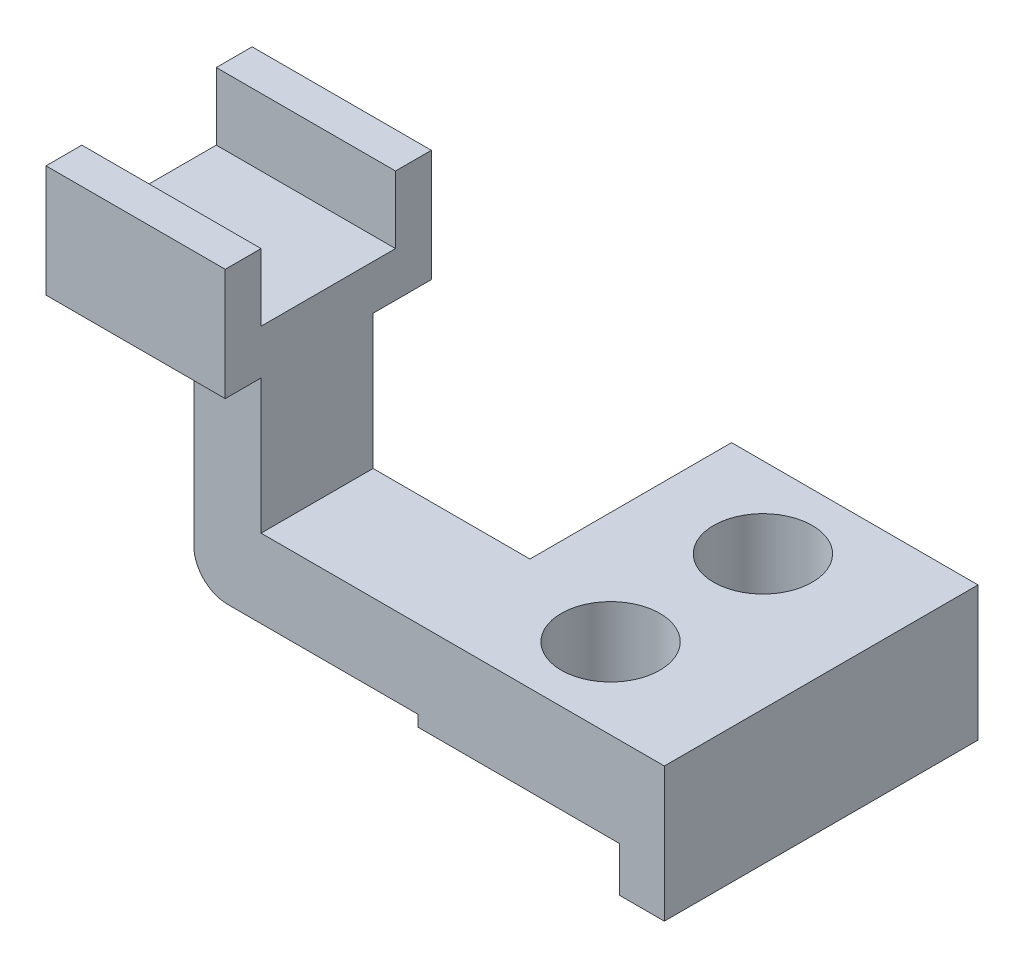
ISO-10303-21;
HEADER;
FILE_DESCRIPTION(('STEP AP214'),'2;1');
FILE_NAME('part.step','',(''),(''),'','','');
FILE_SCHEMA(('AUTOMOTIVE_DESIGN { 1 0 10303 214 1 1 1 1 }'));
ENDSEC;
DATA;
#1=APPLICATION_CONTEXT('core data for automotive mechanical design processes');
#2=APPLICATION_PROTOCOL_DEFINITION('international standard','automotive_design',2000,#1);
#3=PRODUCT_CONTEXT('',#1,'mechanical');
#4=PRODUCT('Part','Part','',(#3));
#5=PRODUCT_RELATED_PRODUCT_CATEGORY('part','',(#4));
#6=PRODUCT_DEFINITION_FORMATION('','',#4);
#7=PRODUCT_DEFINITION_CONTEXT('part definition',#1,'design');
#8=PRODUCT_DEFINITION('design','',#6,#7);
#9=PRODUCT_DEFINITION_SHAPE('','',#8);
#10=(LENGTH_UNIT() NAMED_UNIT(*) SI_UNIT(.MILLI.,.METRE.));
#11=(NAMED_UNIT(*) PLANE_ANGLE_UNIT() SI_UNIT($,.RADIAN.));
#12=(NAMED_UNIT(*) SI_UNIT($,.STERADIAN.) SOLID_ANGLE_UNIT());
#13=UNCERTAINTY_MEASURE_WITH_UNIT(LENGTH_MEASURE(1.E-05),#10,'distance_accuracy_value','');
#14=(GEOMETRIC_REPRESENTATION_CONTEXT(3) GLOBAL_UNCERTAINTY_ASSIGNED_CONTEXT((#13)) GLOBAL_UNIT_ASSIGNED_CONTEXT((#10,
#11,#12)) REPRESENTATION_CONTEXT('',''));
#15=CARTESIAN_POINT('',(0.,0.,0.));
#16=DIRECTION('',(0.,0.,1.));
#17=DIRECTION('',(1.,0.,0.));
#18=AXIS2_PLACEMENT_3D('',#15,#16,#17);
#19=CARTESIAN_POINT('',(0.,20.,70.));
#20=DIRECTION('',(1.,0.,0.));
#21=DIRECTION('',(0.,0.,-1.));
#22=AXIS2_PLACEMENT_3D('',#19,#20,#21);
#23=PLANE('',#22);
#24=DIRECTION('',(0.,0.,1.));
#25=VECTOR('',#24,1.);
#26=CARTESIAN_POINT('',(0.,2.5,45.));
#27=LINE('',#26,#25);
#28=CARTESIAN_POINT('',(0.,2.5,45.));
#29=VERTEX_POINT('',#28);
#30=CARTESIAN_POINT('',(0.,2.5,70.));
#31=VERTEX_POINT('',#30);
#32=EDGE_CURVE('E305',#29,#31,#27,.T.);
#33=ORIENTED_EDGE('',*,*,#32,.F.);
#34=DIRECTION('',(0.,-1.,0.));
#35=VECTOR('',#34,1.);
#36=CARTESIAN_POINT('',(0.,0.,45.));
#37=LINE('',#36,#35);
#38=CARTESIAN_POINT('',(0.,20.,45.));
#39=VERTEX_POINT('',#38);
#40=EDGE_CURVE('E63',#39,#29,#37,.T.);
#41=ORIENTED_EDGE('',*,*,#40,.F.);
#42=DIRECTION('',(0.,0.,-1.));
#43=VECTOR('',#42,1.);
#44=CARTESIAN_POINT('',(0.,20.,70.));
#45=LINE('',#44,#43);
#46=CARTESIAN_POINT('',(0.,20.,0.));
#47=VERTEX_POINT('',#46);
#48=EDGE_CURVE('E317',#39,#47,#45,.T.);
#49=ORIENTED_EDGE('',*,*,#48,.T.);
#50=DIRECTION('',(0.,-1.,0.));
#51=VECTOR('',#50,1.);
#52=CARTESIAN_POINT('',(0.,20.,0.));
#53=LINE('',#52,#51);
#54=CARTESIAN_POINT('',(0.,0.,0.));
#55=VERTEX_POINT('',#54);
#56=EDGE_CURVE('E296',#47,#55,#53,.T.);
#57=ORIENTED_EDGE('',*,*,#56,.T.);
#58=DIRECTION('',(0.,0.,-1.));
#59=VECTOR('',#58,1.);
#60=CARTESIAN_POINT('',(0.,0.,70.));
#61=LINE('',#60,#59);
#62=CARTESIAN_POINT('',(0.,0.,70.));
#63=VERTEX_POINT('',#62);
#64=EDGE_CURVE('E11',#63,#55,#61,.T.);
#65=ORIENTED_EDGE('',*,*,#64,.F.);
#66=DIRECTION('',(0.,-1.,0.));
#67=VECTOR('',#66,1.);
#68=CARTESIAN_POINT('',(0.,20.,70.));
#69=LINE('',#68,#67);
#70=EDGE_CURVE('E70',#31,#63,#69,.T.);
#71=ORIENTED_EDGE('',*,*,#70,.F.);
#72=EDGE_LOOP('',(#33,#41,#49,#57,#65,#71));
#73=FACE_BOUND('',#72,.T.);
#74=ADVANCED_FACE('F50',(#73),#23,.F.);
#75=CARTESIAN_POINT('',(0.,0.,70.));
#76=DIRECTION('',(0.,1.,0.));
#77=DIRECTION('',(0.,0.,1.));
#78=AXIS2_PLACEMENT_3D('',#75,#76,#77);
#79=PLANE('',#78);
#80=CARTESIAN_POINT('',(25.,0.,18.));
#81=DIRECTION('',(0.,1.,0.));
#82=DIRECTION('',(0.,0.,1.));
#83=AXIS2_PLACEMENT_3D('',#80,#81,#82);
#84=CIRCLE('',#83,11.);
#85=CARTESIAN_POINT('',(25.,0.,29.));
#86=VERTEX_POINT('',#85);
#87=EDGE_CURVE('E216',#86,#86,#84,.T.);
#88=ORIENTED_EDGE('',*,*,#87,.T.);
#89=EDGE_LOOP('',(#88));
#90=FACE_BOUND('',#89,.T.);
#91=CARTESIAN_POINT('',(25.,0.,52.));
#92=DIRECTION('',(0.,1.,0.));
#93=DIRECTION('',(0.,0.,1.));
#94=AXIS2_PLACEMENT_3D('',#91,#92,#93);
#95=CIRCLE('',#94,11.);
#96=CARTESIAN_POINT('',(25.,0.,63.));
#97=VERTEX_POINT('',#96);
#98=EDGE_CURVE('E732',#97,#97,#95,.T.);
#99=ORIENTED_EDGE('',*,*,#98,.T.);
#100=EDGE_LOOP('',(#99));
#101=FACE_BOUND('',#100,.T.);
#102=DIRECTION('',(1.,0.,0.));
#103=VECTOR('',#102,1.);
#104=CARTESIAN_POINT('',(0.,0.,0.));
#105=LINE('',#104,#103);
#106=CARTESIAN_POINT('',(45.,0.,0.));
#107=VERTEX_POINT('',#106);
#108=EDGE_CURVE('E325',#55,#107,#105,.T.);
#109=ORIENTED_EDGE('',*,*,#108,.T.);
#110=DIRECTION('',(0.,0.,-1.));
#111=VECTOR('',#110,1.);
#112=CARTESIAN_POINT('',(45.,0.,70.));
#113=LINE('',#112,#111);
#114=CARTESIAN_POINT('',(45.,0.,70.));
#115=VERTEX_POINT('',#114);
#116=EDGE_CURVE('E53',#115,#107,#113,.T.);
#117=ORIENTED_EDGE('',*,*,#116,.F.);
#118=DIRECTION('',(1.,0.,0.));
#119=VECTOR('',#118,1.);
#120=CARTESIAN_POINT('',(0.,0.,70.));
#121=LINE('',#120,#119);
#122=EDGE_CURVE('E306',#63,#115,#121,.T.);
#123=ORIENTED_EDGE('',*,*,#122,.F.);
#124=ORIENTED_EDGE('',*,*,#64,.T.);
#125=EDGE_LOOP('',(#109,#117,#123,#124));
#126=FACE_BOUND('',#125,.T.);
#127=ADVANCED_FACE('F366',(#90,#101,#126),#79,.F.);
#128=CARTESIAN_POINT('',(45.,0.,70.));
#129=DIRECTION('',(1.,0.,0.));
#130=DIRECTION('',(0.,0.,-1.));
#131=AXIS2_PLACEMENT_3D('',#128,#129,#130);
#132=PLANE('',#131);
#133=DIRECTION('',(0.,-1.,0.));
#134=VECTOR('',#133,1.);
#135=CARTESIAN_POINT('',(45.,0.,0.));
#136=LINE('',#135,#134);
#137=CARTESIAN_POINT('',(45.,-10.,0.));
#138=VERTEX_POINT('',#137);
#139=EDGE_CURVE('E322',#107,#138,#136,.T.);
#140=ORIENTED_EDGE('',*,*,#139,.T.);
#141=DIRECTION('',(0.,0.,-1.));
#142=VECTOR('',#141,1.);
#143=CARTESIAN_POINT('',(45.,-10.,70.));
#144=LINE('',#143,#142);
#145=CARTESIAN_POINT('',(45.,-10.,70.));
#146=VERTEX_POINT('',#145);
#147=EDGE_CURVE('E339',#146,#138,#144,.T.);
#148=ORIENTED_EDGE('',*,*,#147,.F.);
#149=DIRECTION('',(0.,-1.,0.));
#150=VECTOR('',#149,1.);
#151=CARTESIAN_POINT('',(45.,0.,70.));
#152=LINE('',#151,#150);
#153=EDGE_CURVE('E313',#115,#146,#152,.T.);
#154=ORIENTED_EDGE('',*,*,#153,.F.);
#155=ORIENTED_EDGE('',*,*,#116,.T.);
#156=EDGE_LOOP('',(#140,#148,#154,#155));
#157=FACE_BOUND('',#156,.T.);
#158=ADVANCED_FACE('F347',(#157),#132,.F.);
#159=CARTESIAN_POINT('',(45.,-10.,70.));
#160=DIRECTION('',(0.,1.,0.));
#161=DIRECTION('',(0.,0.,1.));
#162=AXIS2_PLACEMENT_3D('',#159,#160,#161);
#163=PLANE('',#162);
#164=DIRECTION('',(1.,0.,0.));
#165=VECTOR('',#164,1.);
#166=CARTESIAN_POINT('',(45.,-10.,0.));
#167=LINE('',#166,#165);
#168=CARTESIAN_POINT('',(55.,-10.,0.));
#169=VERTEX_POINT('',#168);
#170=EDGE_CURVE('E326',#138,#169,#167,.T.);
#171=ORIENTED_EDGE('',*,*,#170,.T.);
#172=DIRECTION('',(0.,0.,-1.));
#173=VECTOR('',#172,1.);
#174=CARTESIAN_POINT('',(55.,-10.,70.));
#175=LINE('',#174,#173);
#176=CARTESIAN_POINT('',(55.,-10.,70.));
#177=VERTEX_POINT('',#176);
#178=EDGE_CURVE('E338',#177,#169,#175,.T.);
#179=ORIENTED_EDGE('',*,*,#178,.F.);
#180=DIRECTION('',(1.,0.,0.));
#181=VECTOR('',#180,1.);
#182=CARTESIAN_POINT('',(45.,-10.,70.));
#183=LINE('',#182,#181);
#184=EDGE_CURVE('E311',#146,#177,#183,.T.);
#185=ORIENTED_EDGE('',*,*,#184,.F.);
#186=ORIENTED_EDGE('',*,*,#147,.T.);
#187=EDGE_LOOP('',(#171,#179,#185,#186));
#188=FACE_BOUND('',#187,.T.);
#189=ADVANCED_FACE('F356',(#188),#163,.F.);
#190=CARTESIAN_POINT('',(55.,-10.,70.));
#191=DIRECTION('',(-1.,0.,0.));
#192=DIRECTION('',(0.,0.,1.));
#193=AXIS2_PLACEMENT_3D('',#190,#191,#192);
#194=PLANE('',#193);
#195=DIRECTION('',(0.,1.,0.));
#196=VECTOR('',#195,1.);
#197=CARTESIAN_POINT('',(55.,-10.,0.));
#198=LINE('',#197,#196);
#199=CARTESIAN_POINT('',(55.,20.,0.));
#200=VERTEX_POINT('',#199);
#201=EDGE_CURVE('E327',#169,#200,#198,.T.);
#202=ORIENTED_EDGE('',*,*,#201,.T.);
#203=DIRECTION('',(0.,0.,-1.));
#204=VECTOR('',#203,1.);
#205=CARTESIAN_POINT('',(55.,20.,70.));
#206=LINE('',#205,#204);
#207=CARTESIAN_POINT('',(55.,20.,70.));
#208=VERTEX_POINT('',#207);
#209=EDGE_CURVE('E334',#208,#200,#206,.T.);
#210=ORIENTED_EDGE('',*,*,#209,.F.);
#211=DIRECTION('',(0.,1.,0.));
#212=VECTOR('',#211,1.);
#213=CARTESIAN_POINT('',(55.,-10.,70.));
#214=LINE('',#213,#212);
#215=EDGE_CURVE('E312',#177,#208,#214,.T.);
#216=ORIENTED_EDGE('',*,*,#215,.F.);
#217=ORIENTED_EDGE('',*,*,#178,.T.);
#218=EDGE_LOOP('',(#202,#210,#216,#217));
#219=FACE_BOUND('',#218,.T.);
#220=ADVANCED_FACE('F362',(#219),#194,.F.);
#221=CARTESIAN_POINT('',(55.,20.,70.));
#222=DIRECTION('',(0.,-1.,0.));
#223=DIRECTION('',(0.,0.,-1.));
#224=AXIS2_PLACEMENT_3D('',#221,#222,#223);
#225=PLANE('',#224);
#226=CARTESIAN_POINT('',(25.,20.,18.));
#227=DIRECTION('',(0.,1.,0.));
#228=DIRECTION('',(0.,0.,1.));
#229=AXIS2_PLACEMENT_3D('',#226,#227,#228);
#230=CIRCLE('',#229,11.);
#231=CARTESIAN_POINT('',(25.,20.,29.));
#232=VERTEX_POINT('',#231);
#233=EDGE_CURVE('E729',#232,#232,#230,.T.);
#234=ORIENTED_EDGE('',*,*,#233,.F.);
#235=EDGE_LOOP('',(#234));
#236=FACE_BOUND('',#235,.T.);
#237=CARTESIAN_POINT('',(25.,20.,52.));
#238=DIRECTION('',(0.,1.,0.));
#239=DIRECTION('',(0.,0.,1.));
#240=AXIS2_PLACEMENT_3D('',#237,#238,#239);
#241=CIRCLE('',#240,11.);
#242=CARTESIAN_POINT('',(25.,20.,63.));
#243=VERTEX_POINT('',#242);
#244=EDGE_CURVE('E734',#243,#243,#241,.T.);
#245=ORIENTED_EDGE('',*,*,#244,.F.);
#246=EDGE_LOOP('',(#245));
#247=FACE_BOUND('',#246,.T.);
#248=DIRECTION('',(-1.,0.,0.));
#249=VECTOR('',#248,1.);
#250=CARTESIAN_POINT('',(55.,20.,0.));
#251=LINE('',#250,#249);
#252=EDGE_CURVE('E310',#200,#47,#251,.T.);
#253=ORIENTED_EDGE('',*,*,#252,.T.);
#254=ORIENTED_EDGE('',*,*,#48,.F.);
#255=DIRECTION('',(-1.,0.,0.));
#256=VECTOR('',#255,1.);
#257=CARTESIAN_POINT('',(0.,20.,45.));
#258=LINE('',#257,#256);
#259=CARTESIAN_POINT('',(-35.,20.,45.));
#260=VERTEX_POINT('',#259);
#261=EDGE_CURVE('E274',#39,#260,#258,.T.);
#262=ORIENTED_EDGE('',*,*,#261,.T.);
#263=DIRECTION('',(0.,0.,1.));
#264=VECTOR('',#263,1.);
#265=CARTESIAN_POINT('',(-35.,20.,45.));
#266=LINE('',#265,#264);
#267=CARTESIAN_POINT('',(-35.,20.,70.));
#268=VERTEX_POINT('',#267);
#269=EDGE_CURVE('E299',#260,#268,#266,.T.);
#270=ORIENTED_EDGE('',*,*,#269,.T.);
#271=DIRECTION('',(-1.,0.,0.));
#272=VECTOR('',#271,1.);
#273=CARTESIAN_POINT('',(55.,20.,70.));
#274=LINE('',#273,#272);
#275=EDGE_CURVE('E320',#208,#268,#274,.T.);
#276=ORIENTED_EDGE('',*,*,#275,.F.);
#277=ORIENTED_EDGE('',*,*,#209,.T.);
#278=EDGE_LOOP('',(#253,#254,#262,#270,#276,#277));
#279=FACE_BOUND('',#278,.T.);
#280=ADVANCED_FACE('F367',(#236,#247,#279),#225,.F.);
#281=CARTESIAN_POINT('',(0.,0.,70.));
#282=DIRECTION('',(0.,0.,1.));
#283=DIRECTION('',(1.,0.,0.));
#284=AXIS2_PLACEMENT_3D('',#281,#282,#283);
#285=PLANE('',#284);
#286=ORIENTED_EDGE('',*,*,#275,.T.);
#287=DIRECTION('',(0.,1.,0.));
#288=VECTOR('',#287,1.);
#289=CARTESIAN_POINT('',(-35.,0.,70.));
#290=LINE('',#289,#288);
#291=CARTESIAN_POINT('',(-35.,50.,70.));
#292=VERTEX_POINT('',#291);
#293=EDGE_CURVE('E295',#268,#292,#290,.T.);
#294=ORIENTED_EDGE('',*,*,#293,.T.);
#295=DIRECTION('',(-1.,0.,0.));
#296=VECTOR('',#295,1.);
#297=CARTESIAN_POINT('',(0.,50.,70.));
#298=LINE('',#297,#296);
#299=CARTESIAN_POINT('',(-50.,50.,70.));
#300=VERTEX_POINT('',#299);
#301=EDGE_CURVE('E267',#292,#300,#298,.T.);
#302=ORIENTED_EDGE('',*,*,#301,.T.);
#303=DIRECTION('',(0.,-1.,0.));
#304=VECTOR('',#303,1.);
#305=CARTESIAN_POINT('',(-50.,0.,70.));
#306=LINE('',#305,#304);
#307=CARTESIAN_POINT('',(-50.,9.99999999999999,70.));
#308=VERTEX_POINT('',#307);
#309=EDGE_CURVE('E251',#300,#308,#306,.T.);
#310=ORIENTED_EDGE('',*,*,#309,.T.);
#311=CARTESIAN_POINT('',(-42.5,9.99999999999999,70.));
#312=DIRECTION('',(0.,0.,1.));
#313=DIRECTION('',(1.,0.,0.));
#314=AXIS2_PLACEMENT_3D('',#311,#312,#313);
#315=CIRCLE('',#314,7.50000000000001);
#316=CARTESIAN_POINT('',(-42.5,2.49999999999999,70.));
#317=VERTEX_POINT('',#316);
#318=EDGE_CURVE('E288',#308,#317,#315,.T.);
#319=ORIENTED_EDGE('',*,*,#318,.T.);
#320=DIRECTION('',(-1.,0.,0.));
#321=VECTOR('',#320,1.);
#322=CARTESIAN_POINT('',(0.,2.5,70.));
#323=LINE('',#322,#321);
#324=EDGE_CURVE('E289',#31,#317,#323,.T.);
#325=ORIENTED_EDGE('',*,*,#324,.F.);
#326=ORIENTED_EDGE('',*,*,#70,.T.);
#327=ORIENTED_EDGE('',*,*,#122,.T.);
#328=ORIENTED_EDGE('',*,*,#153,.T.);
#329=ORIENTED_EDGE('',*,*,#184,.T.);
#330=ORIENTED_EDGE('',*,*,#215,.T.);
#331=EDGE_LOOP('',(#286,#294,#302,#310,#319,#325,#326,#327,#328,#329,#330));
#332=FACE_BOUND('',#331,.T.);
#333=ADVANCED_FACE('F368',(#332),#285,.T.);
#334=CARTESIAN_POINT('',(0.,0.,0.));
#335=DIRECTION('',(0.,0.,1.));
#336=DIRECTION('',(1.,0.,0.));
#337=AXIS2_PLACEMENT_3D('',#334,#335,#336);
#338=PLANE('',#337);
#339=ORIENTED_EDGE('',*,*,#56,.F.);
#340=ORIENTED_EDGE('',*,*,#252,.F.);
#341=ORIENTED_EDGE('',*,*,#201,.F.);
#342=ORIENTED_EDGE('',*,*,#170,.F.);
#343=ORIENTED_EDGE('',*,*,#139,.F.);
#344=ORIENTED_EDGE('',*,*,#108,.F.);
#345=EDGE_LOOP('',(#339,#340,#341,#342,#343,#344));
#346=FACE_BOUND('',#345,.T.);
#347=ADVANCED_FACE('F351',(#346),#338,.F.);
#348=CARTESIAN_POINT('',(-50.,0.,45.));
#349=DIRECTION('',(-1.,0.,0.));
#350=DIRECTION('',(0.,0.,1.));
#351=AXIS2_PLACEMENT_3D('',#348,#349,#350);
#352=PLANE('',#351);
#353=ORIENTED_EDGE('',*,*,#309,.F.);
#354=DIRECTION('',(0.,0.,1.));
#355=VECTOR('',#354,1.);
#356=CARTESIAN_POINT('',(-50.,50.,45.));
#357=LINE('',#356,#355);
#358=CARTESIAN_POINT('',(-50.,50.,45.));
#359=VERTEX_POINT('',#358);
#360=EDGE_CURVE('E293',#359,#300,#357,.T.);
#361=ORIENTED_EDGE('',*,*,#360,.F.);
#362=DIRECTION('',(0.,-1.,0.));
#363=VECTOR('',#362,1.);
#364=CARTESIAN_POINT('',(-50.,0.,45.));
#365=LINE('',#364,#363);
#366=CARTESIAN_POINT('',(-50.,9.99999999999999,45.));
#367=VERTEX_POINT('',#366);
#368=EDGE_CURVE('E264',#359,#367,#365,.T.);
#369=ORIENTED_EDGE('',*,*,#368,.T.);
#370=DIRECTION('',(0.,0.,1.));
#371=VECTOR('',#370,1.);
#372=CARTESIAN_POINT('',(-50.,9.99999999999999,45.));
#373=LINE('',#372,#371);
#374=EDGE_CURVE('E281',#367,#308,#373,.T.);
#375=ORIENTED_EDGE('',*,*,#374,.T.);
#376=EDGE_LOOP('',(#353,#361,#369,#375));
#377=FACE_BOUND('',#376,.T.);
#378=ADVANCED_FACE('F379',(#377),#352,.T.);
#379=CARTESIAN_POINT('',(-35.,0.,45.));
#380=DIRECTION('',(1.,0.,0.));
#381=DIRECTION('',(0.,0.,-1.));
#382=AXIS2_PLACEMENT_3D('',#379,#380,#381);
#383=PLANE('',#382);
#384=ORIENTED_EDGE('',*,*,#293,.F.);
#385=ORIENTED_EDGE('',*,*,#269,.F.);
#386=DIRECTION('',(0.,1.,0.));
#387=VECTOR('',#386,1.);
#388=CARTESIAN_POINT('',(-35.,0.,45.));
#389=LINE('',#388,#387);
#390=CARTESIAN_POINT('',(-35.,50.,45.));
#391=VERTEX_POINT('',#390);
#392=EDGE_CURVE('E279',#260,#391,#389,.T.);
#393=ORIENTED_EDGE('',*,*,#392,.T.);
#394=DIRECTION('',(0.,0.,-1.));
#395=VECTOR('',#394,1.);
#396=CARTESIAN_POINT('',(-35.,50.,70.));
#397=LINE('',#396,#395);
#398=CARTESIAN_POINT('',(-35.,50.,32.));
#399=VERTEX_POINT('',#398);
#400=EDGE_CURVE('E213',#391,#399,#397,.T.);
#401=ORIENTED_EDGE('',*,*,#400,.T.);
#402=DIRECTION('',(0.,1.,0.));
#403=VECTOR('',#402,1.);
#404=CARTESIAN_POINT('',(-35.,75.,32.));
#405=LINE('',#404,#403);
#406=CARTESIAN_POINT('',(-35.,75.,32.));
#407=VERTEX_POINT('',#406);
#408=EDGE_CURVE('E186',#399,#407,#405,.T.);
#409=ORIENTED_EDGE('',*,*,#408,.T.);
#410=DIRECTION('',(0.,0.,1.));
#411=VECTOR('',#410,1.);
#412=CARTESIAN_POINT('',(-35.,75.,40.));
#413=LINE('',#412,#411);
#414=CARTESIAN_POINT('',(-35.,75.,40.));
#415=VERTEX_POINT('',#414);
#416=EDGE_CURVE('E234',#407,#415,#413,.T.);
#417=ORIENTED_EDGE('',*,*,#416,.T.);
#418=DIRECTION('',(0.,-1.,0.));
#419=VECTOR('',#418,1.);
#420=CARTESIAN_POINT('',(-35.,60.,40.));
#421=LINE('',#420,#419);
#422=CARTESIAN_POINT('',(-35.,60.,40.));
#423=VERTEX_POINT('',#422);
#424=EDGE_CURVE('E240',#415,#423,#421,.T.);
#425=ORIENTED_EDGE('',*,*,#424,.T.);
#426=DIRECTION('',(0.,0.,1.));
#427=VECTOR('',#426,1.);
#428=CARTESIAN_POINT('',(-35.,60.,70.));
#429=LINE('',#428,#427);
#430=CARTESIAN_POINT('',(-35.,60.,70.));
#431=VERTEX_POINT('',#430);
#432=EDGE_CURVE('E238',#423,#431,#429,.T.);
#433=ORIENTED_EDGE('',*,*,#432,.T.);
#434=DIRECTION('',(0.,1.,0.));
#435=VECTOR('',#434,1.);
#436=CARTESIAN_POINT('',(-35.,75.,70.));
#437=LINE('',#436,#435);
#438=CARTESIAN_POINT('',(-35.,75.,70.));
#439=VERTEX_POINT('',#438);
#440=EDGE_CURVE('E241',#431,#439,#437,.T.);
#441=ORIENTED_EDGE('',*,*,#440,.T.);
#442=DIRECTION('',(0.,0.,1.));
#443=VECTOR('',#442,1.);
#444=CARTESIAN_POINT('',(-35.,75.,78.));
#445=LINE('',#444,#443);
#446=CARTESIAN_POINT('',(-35.,75.,78.));
#447=VERTEX_POINT('',#446);
#448=EDGE_CURVE('E248',#439,#447,#445,.T.);
#449=ORIENTED_EDGE('',*,*,#448,.T.);
#450=DIRECTION('',(0.,-1.,0.));
#451=VECTOR('',#450,1.);
#452=CARTESIAN_POINT('',(-35.,50.,78.));
#453=LINE('',#452,#451);
#454=CARTESIAN_POINT('',(-35.,50.,78.));
#455=VERTEX_POINT('',#454);
#456=EDGE_CURVE('E249',#447,#455,#453,.T.);
#457=ORIENTED_EDGE('',*,*,#456,.T.);
#458=EDGE_CURVE('E209',#455,#292,#397,.T.);
#459=ORIENTED_EDGE('',*,*,#458,.T.);
#460=EDGE_LOOP('',(#384,#385,#393,#401,#409,#417,#425,#433,#441,#449,#457,#459));
#461=FACE_BOUND('',#460,.T.);
#462=ADVANCED_FACE('F374',(#461),#383,.T.);
#463=CARTESIAN_POINT('',(0.,2.5,45.));
#464=DIRECTION('',(0.,1.,0.));
#465=DIRECTION('',(-1.,0.,0.));
#466=AXIS2_PLACEMENT_3D('',#463,#464,#465);
#467=PLANE('',#466);
#468=ORIENTED_EDGE('',*,*,#324,.T.);
#469=DIRECTION('',(0.,0.,1.));
#470=VECTOR('',#469,1.);
#471=CARTESIAN_POINT('',(-42.5,2.49999999999999,45.));
#472=LINE('',#471,#470);
#473=CARTESIAN_POINT('',(-42.5,2.49999999999999,45.));
#474=VERTEX_POINT('',#473);
#475=EDGE_CURVE('E304',#474,#317,#472,.T.);
#476=ORIENTED_EDGE('',*,*,#475,.F.);
#477=DIRECTION('',(-1.,0.,0.));
#478=VECTOR('',#477,1.);
#479=CARTESIAN_POINT('',(0.,2.5,45.));
#480=LINE('',#479,#478);
#481=EDGE_CURVE('E275',#29,#474,#480,.T.);
#482=ORIENTED_EDGE('',*,*,#481,.F.);
#483=ORIENTED_EDGE('',*,*,#32,.T.);
#484=EDGE_LOOP('',(#468,#476,#482,#483));
#485=FACE_BOUND('',#484,.T.);
#486=ADVANCED_FACE('F388',(#485),#467,.F.);
#487=CARTESIAN_POINT('',(-42.5,9.99999999999999,45.));
#488=DIRECTION('',(0.,0.,1.));
#489=DIRECTION('',(1.,0.,0.));
#490=AXIS2_PLACEMENT_3D('',#487,#488,#489);
#491=CYLINDRICAL_SURFACE('',#490,7.50000000000001);
#492=ORIENTED_EDGE('',*,*,#318,.F.);
#493=ORIENTED_EDGE('',*,*,#374,.F.);
#494=CARTESIAN_POINT('',(-42.5,9.99999999999999,45.));
#495=DIRECTION('',(0.,0.,1.));
#496=DIRECTION('',(1.,0.,0.));
#497=AXIS2_PLACEMENT_3D('',#494,#495,#496);
#498=CIRCLE('',#497,7.50000000000001);
#499=EDGE_CURVE('E268',#367,#474,#498,.T.);
#500=ORIENTED_EDGE('',*,*,#499,.T.);
#501=ORIENTED_EDGE('',*,*,#475,.T.);
#502=EDGE_LOOP('',(#492,#493,#500,#501));
#503=FACE_BOUND('',#502,.T.);
#504=ADVANCED_FACE('F389',(#503),#491,.T.);
#505=CARTESIAN_POINT('',(0.,0.,45.));
#506=DIRECTION('',(0.,0.,1.));
#507=DIRECTION('',(1.,0.,0.));
#508=AXIS2_PLACEMENT_3D('',#505,#506,#507);
#509=PLANE('',#508);
#510=ORIENTED_EDGE('',*,*,#368,.F.);
#511=DIRECTION('',(-1.,0.,0.));
#512=VECTOR('',#511,1.);
#513=CARTESIAN_POINT('',(0.,50.,45.));
#514=LINE('',#513,#512);
#515=EDGE_CURVE('E278',#391,#359,#514,.T.);
#516=ORIENTED_EDGE('',*,*,#515,.F.);
#517=ORIENTED_EDGE('',*,*,#392,.F.);
#518=ORIENTED_EDGE('',*,*,#261,.F.);
#519=ORIENTED_EDGE('',*,*,#40,.T.);
#520=ORIENTED_EDGE('',*,*,#481,.T.);
#521=ORIENTED_EDGE('',*,*,#499,.F.);
#522=EDGE_LOOP('',(#510,#516,#517,#518,#519,#520,#521));
#523=FACE_BOUND('',#522,.T.);
#524=ADVANCED_FACE('F382',(#523),#509,.F.);
#525=CARTESIAN_POINT('',(-75.,50.,70.));
#526=DIRECTION('',(0.,-1.,0.));
#527=DIRECTION('',(0.,0.,-1.));
#528=AXIS2_PLACEMENT_3D('',#525,#526,#527);
#529=PLANE('',#528);
#530=ORIENTED_EDGE('',*,*,#301,.F.);
#531=ORIENTED_EDGE('',*,*,#458,.F.);
#532=DIRECTION('',(1.,0.,0.));
#533=VECTOR('',#532,1.);
#534=CARTESIAN_POINT('',(-75.,50.,78.));
#535=LINE('',#534,#533);
#536=CARTESIAN_POINT('',(-75.,50.,78.));
#537=VERTEX_POINT('',#536);
#538=EDGE_CURVE('E208',#537,#455,#535,.T.);
#539=ORIENTED_EDGE('',*,*,#538,.F.);
#540=DIRECTION('',(0.,0.,-1.));
#541=VECTOR('',#540,1.);
#542=CARTESIAN_POINT('',(-75.,50.,32.));
#543=LINE('',#542,#541);
#544=CARTESIAN_POINT('',(-75.,50.,32.));
#545=VERTEX_POINT('',#544);
#546=EDGE_CURVE('E200',#537,#545,#543,.T.);
#547=ORIENTED_EDGE('',*,*,#546,.T.);
#548=DIRECTION('',(1.,0.,0.));
#549=VECTOR('',#548,1.);
#550=CARTESIAN_POINT('',(-75.,50.,32.));
#551=LINE('',#550,#549);
#552=EDGE_CURVE('E181',#545,#399,#551,.T.);
#553=ORIENTED_EDGE('',*,*,#552,.T.);
#554=ORIENTED_EDGE('',*,*,#400,.F.);
#555=ORIENTED_EDGE('',*,*,#515,.T.);
#556=ORIENTED_EDGE('',*,*,#360,.T.);
#557=EDGE_LOOP('',(#530,#531,#539,#547,#553,#554,#555,#556));
#558=FACE_BOUND('',#557,.T.);
#559=ADVANCED_FACE('F206',(#558),#529,.T.);
#560=CARTESIAN_POINT('',(-75.,50.,78.));
#561=DIRECTION('',(0.,0.,1.));
#562=DIRECTION('',(1.,0.,0.));
#563=AXIS2_PLACEMENT_3D('',#560,#561,#562);
#564=PLANE('',#563);
#565=ORIENTED_EDGE('',*,*,#456,.F.);
#566=DIRECTION('',(1.,0.,0.));
#567=VECTOR('',#566,1.);
#568=CARTESIAN_POINT('',(-75.,75.,78.));
#569=LINE('',#568,#567);
#570=CARTESIAN_POINT('',(-75.,75.,78.));
#571=VERTEX_POINT('',#570);
#572=EDGE_CURVE('E255',#571,#447,#569,.T.);
#573=ORIENTED_EDGE('',*,*,#572,.F.);
#574=DIRECTION('',(0.,-1.,0.));
#575=VECTOR('',#574,1.);
#576=CARTESIAN_POINT('',(-75.,50.,78.));
#577=LINE('',#576,#575);
#578=EDGE_CURVE('E191',#571,#537,#577,.T.);
#579=ORIENTED_EDGE('',*,*,#578,.T.);
#580=ORIENTED_EDGE('',*,*,#538,.T.);
#581=EDGE_LOOP('',(#565,#573,#579,#580));
#582=FACE_BOUND('',#581,.T.);
#583=ADVANCED_FACE('F413',(#582),#564,.T.);
#584=CARTESIAN_POINT('',(-75.,75.,78.));
#585=DIRECTION('',(0.,1.,0.));
#586=DIRECTION('',(0.,0.,1.));
#587=AXIS2_PLACEMENT_3D('',#584,#585,#586);
#588=PLANE('',#587);
#589=ORIENTED_EDGE('',*,*,#448,.F.);
#590=DIRECTION('',(1.,0.,0.));
#591=VECTOR('',#590,1.);
#592=CARTESIAN_POINT('',(-75.,75.,70.));
#593=LINE('',#592,#591);
#594=CARTESIAN_POINT('',(-75.,75.,70.));
#595=VERTEX_POINT('',#594);
#596=EDGE_CURVE('E258',#595,#439,#593,.T.);
#597=ORIENTED_EDGE('',*,*,#596,.F.);
#598=DIRECTION('',(0.,0.,1.));
#599=VECTOR('',#598,1.);
#600=CARTESIAN_POINT('',(-75.,75.,78.));
#601=LINE('',#600,#599);
#602=EDGE_CURVE('E229',#595,#571,#601,.T.);
#603=ORIENTED_EDGE('',*,*,#602,.T.);
#604=ORIENTED_EDGE('',*,*,#572,.T.);
#605=EDGE_LOOP('',(#589,#597,#603,#604));
#606=FACE_BOUND('',#605,.T.);
#607=ADVANCED_FACE('F406',(#606),#588,.T.);
#608=CARTESIAN_POINT('',(-75.,75.,70.));
#609=DIRECTION('',(0.,0.,-1.));
#610=DIRECTION('',(-1.,0.,0.));
#611=AXIS2_PLACEMENT_3D('',#608,#609,#610);
#612=PLANE('',#611);
#613=ORIENTED_EDGE('',*,*,#440,.F.);
#614=DIRECTION('',(1.,0.,0.));
#615=VECTOR('',#614,1.);
#616=CARTESIAN_POINT('',(-75.,60.,70.));
#617=LINE('',#616,#615);
#618=CARTESIAN_POINT('',(-75.,60.,70.));
#619=VERTEX_POINT('',#618);
#620=EDGE_CURVE('E256',#619,#431,#617,.T.);
#621=ORIENTED_EDGE('',*,*,#620,.F.);
#622=DIRECTION('',(0.,1.,0.));
#623=VECTOR('',#622,1.);
#624=CARTESIAN_POINT('',(-75.,75.,70.));
#625=LINE('',#624,#623);
#626=EDGE_CURVE('E228',#619,#595,#625,.T.);
#627=ORIENTED_EDGE('',*,*,#626,.T.);
#628=ORIENTED_EDGE('',*,*,#596,.T.);
#629=EDGE_LOOP('',(#613,#621,#627,#628));
#630=FACE_BOUND('',#629,.T.);
#631=ADVANCED_FACE('F404',(#630),#612,.T.);
#632=CARTESIAN_POINT('',(-75.,60.,70.));
#633=DIRECTION('',(0.,1.,0.));
#634=DIRECTION('',(0.,0.,1.));
#635=AXIS2_PLACEMENT_3D('',#632,#633,#634);
#636=PLANE('',#635);
#637=ORIENTED_EDGE('',*,*,#432,.F.);
#638=DIRECTION('',(1.,0.,0.));
#639=VECTOR('',#638,1.);
#640=CARTESIAN_POINT('',(-75.,60.,40.));
#641=LINE('',#640,#639);
#642=CARTESIAN_POINT('',(-75.,60.,40.));
#643=VERTEX_POINT('',#642);
#644=EDGE_CURVE('E257',#643,#423,#641,.T.);
#645=ORIENTED_EDGE('',*,*,#644,.F.);
#646=DIRECTION('',(0.,0.,1.));
#647=VECTOR('',#646,1.);
#648=CARTESIAN_POINT('',(-75.,60.,70.));
#649=LINE('',#648,#647);
#650=EDGE_CURVE('E224',#643,#619,#649,.T.);
#651=ORIENTED_EDGE('',*,*,#650,.T.);
#652=ORIENTED_EDGE('',*,*,#620,.T.);
#653=EDGE_LOOP('',(#637,#645,#651,#652));
#654=FACE_BOUND('',#653,.T.);
#655=ADVANCED_FACE('F397',(#654),#636,.T.);
#656=CARTESIAN_POINT('',(-75.,60.,40.));
#657=DIRECTION('',(0.,0.,1.));
#658=DIRECTION('',(1.,0.,0.));
#659=AXIS2_PLACEMENT_3D('',#656,#657,#658);
#660=PLANE('',#659);
#661=ORIENTED_EDGE('',*,*,#424,.F.);
#662=DIRECTION('',(1.,0.,0.));
#663=VECTOR('',#662,1.);
#664=CARTESIAN_POINT('',(-75.,75.,40.));
#665=LINE('',#664,#663);
#666=CARTESIAN_POINT('',(-75.,75.,40.));
#667=VERTEX_POINT('',#666);
#668=EDGE_CURVE('E265',#667,#415,#665,.T.);
#669=ORIENTED_EDGE('',*,*,#668,.F.);
#670=DIRECTION('',(0.,-1.,0.));
#671=VECTOR('',#670,1.);
#672=CARTESIAN_POINT('',(-75.,60.,40.));
#673=LINE('',#672,#671);
#674=EDGE_CURVE('E219',#667,#643,#673,.T.);
#675=ORIENTED_EDGE('',*,*,#674,.T.);
#676=ORIENTED_EDGE('',*,*,#644,.T.);
#677=EDGE_LOOP('',(#661,#669,#675,#676));
#678=FACE_BOUND('',#677,.T.);
#679=ADVANCED_FACE('F398',(#678),#660,.T.);
#680=CARTESIAN_POINT('',(-75.,75.,40.));
#681=DIRECTION('',(0.,1.,0.));
#682=DIRECTION('',(0.,0.,1.));
#683=AXIS2_PLACEMENT_3D('',#680,#681,#682);
#684=PLANE('',#683);
#685=ORIENTED_EDGE('',*,*,#416,.F.);
#686=DIRECTION('',(1.,0.,0.));
#687=VECTOR('',#686,1.);
#688=CARTESIAN_POINT('',(-75.,75.,32.));
#689=LINE('',#688,#687);
#690=CARTESIAN_POINT('',(-75.,75.,32.));
#691=VERTEX_POINT('',#690);
#692=EDGE_CURVE('E195',#691,#407,#689,.T.);
#693=ORIENTED_EDGE('',*,*,#692,.F.);
#694=DIRECTION('',(0.,0.,1.));
#695=VECTOR('',#694,1.);
#696=CARTESIAN_POINT('',(-75.,75.,40.));
#697=LINE('',#696,#695);
#698=EDGE_CURVE('E201',#691,#667,#697,.T.);
#699=ORIENTED_EDGE('',*,*,#698,.T.);
#700=ORIENTED_EDGE('',*,*,#668,.T.);
#701=EDGE_LOOP('',(#685,#693,#699,#700));
#702=FACE_BOUND('',#701,.T.);
#703=ADVANCED_FACE('F394',(#702),#684,.T.);
#704=CARTESIAN_POINT('',(-75.,75.,32.));
#705=DIRECTION('',(0.,0.,-1.));
#706=DIRECTION('',(-1.,0.,0.));
#707=AXIS2_PLACEMENT_3D('',#704,#705,#706);
#708=PLANE('',#707);
#709=ORIENTED_EDGE('',*,*,#408,.F.);
#710=ORIENTED_EDGE('',*,*,#552,.F.);
#711=DIRECTION('',(0.,1.,0.));
#712=VECTOR('',#711,1.);
#713=CARTESIAN_POINT('',(-75.,75.,32.));
#714=LINE('',#713,#712);
#715=EDGE_CURVE('E188',#545,#691,#714,.T.);
#716=ORIENTED_EDGE('',*,*,#715,.T.);
#717=ORIENTED_EDGE('',*,*,#692,.T.);
#718=EDGE_LOOP('',(#709,#710,#716,#717));
#719=FACE_BOUND('',#718,.T.);
#720=ADVANCED_FACE('F183',(#719),#708,.T.);
#721=CARTESIAN_POINT('',(-75.,0.,0.));
#722=DIRECTION('',(-1.,0.,0.));
#723=DIRECTION('',(0.,0.,1.));
#724=AXIS2_PLACEMENT_3D('',#721,#722,#723);
#725=PLANE('',#724);
#726=ORIENTED_EDGE('',*,*,#546,.F.);
#727=ORIENTED_EDGE('',*,*,#578,.F.);
#728=ORIENTED_EDGE('',*,*,#602,.F.);
#729=ORIENTED_EDGE('',*,*,#626,.F.);
#730=ORIENTED_EDGE('',*,*,#650,.F.);
#731=ORIENTED_EDGE('',*,*,#674,.F.);
#732=ORIENTED_EDGE('',*,*,#698,.F.);
#733=ORIENTED_EDGE('',*,*,#715,.F.);
#734=EDGE_LOOP('',(#726,#727,#728,#729,#730,#731,#732,#733));
#735=FACE_BOUND('',#734,.T.);
#736=ADVANCED_FACE('F197',(#735),#725,.T.);
#737=CARTESIAN_POINT('',(25.,-10.,52.));
#738=DIRECTION('',(0.,1.,0.));
#739=DIRECTION('',(0.,0.,1.));
#740=AXIS2_PLACEMENT_3D('',#737,#738,#739);
#741=CYLINDRICAL_SURFACE('',#740,11.);
#742=ORIENTED_EDGE('',*,*,#244,.T.);
#743=EDGE_LOOP('',(#742));
#744=FACE_BOUND('',#743,.T.);
#745=ORIENTED_EDGE('',*,*,#98,.F.);
#746=EDGE_LOOP('',(#745));
#747=FACE_BOUND('',#746,.T.);
#748=ADVANCED_FACE('F487',(#744,#747),#741,.F.);
#749=CARTESIAN_POINT('',(25.,-10.,18.));
#750=DIRECTION('',(0.,1.,0.));
#751=DIRECTION('',(0.,0.,1.));
#752=AXIS2_PLACEMENT_3D('',#749,#750,#751);
#753=CYLINDRICAL_SURFACE('',#752,11.);
#754=ORIENTED_EDGE('',*,*,#233,.T.);
#755=EDGE_LOOP('',(#754));
#756=FACE_BOUND('',#755,.T.);
#757=ORIENTED_EDGE('',*,*,#87,.F.);
#758=EDGE_LOOP('',(#757));
#759=FACE_BOUND('',#758,.T.);
#760=ADVANCED_FACE('F494',(#756,#759),#753,.F.);
#761=CLOSED_SHELL('',(#74,#127,#158,#189,#220,#280,#333,#347,#378,#462,#486,#504,#524,#559,#583,
#607,#631,#655,#679,#703,#720,#736,#748,#760));
#762=MANIFOLD_SOLID_BREP('B2',#761);
#763=ADVANCED_BREP_SHAPE_REPRESENTATION('',(#18,#762),#14);
#764=SHAPE_DEFINITION_REPRESENTATION(#9,#763);
ENDSEC;
END-ISO-10303-21;
